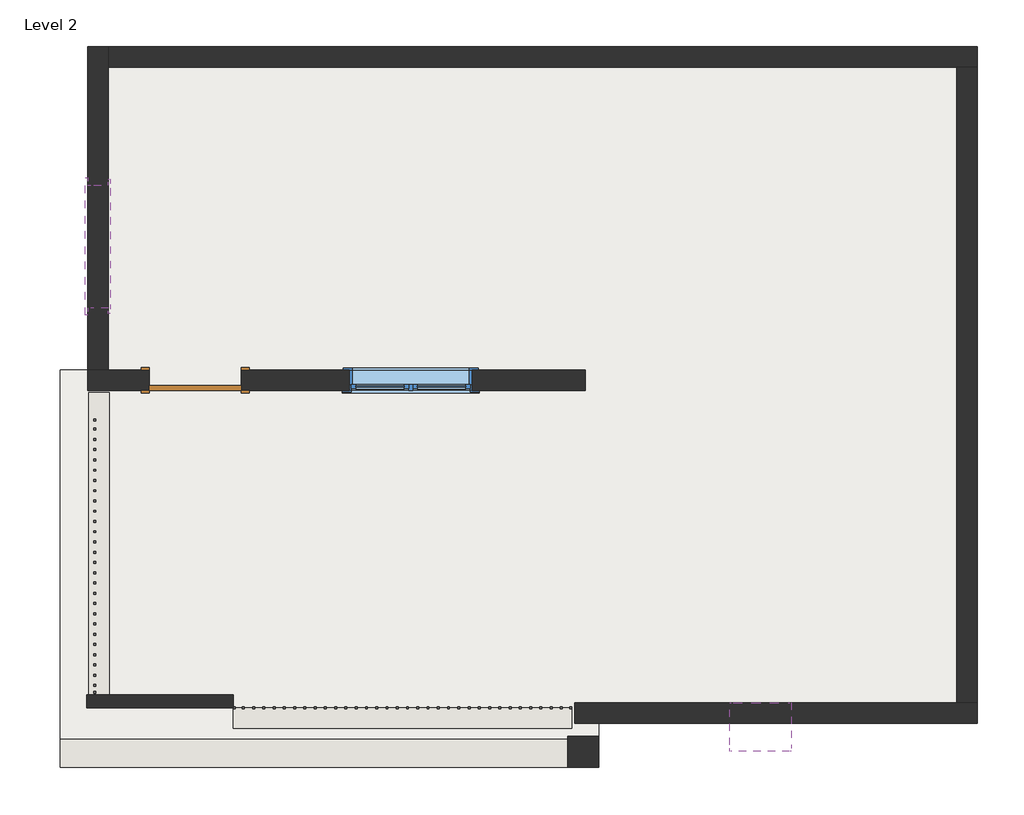
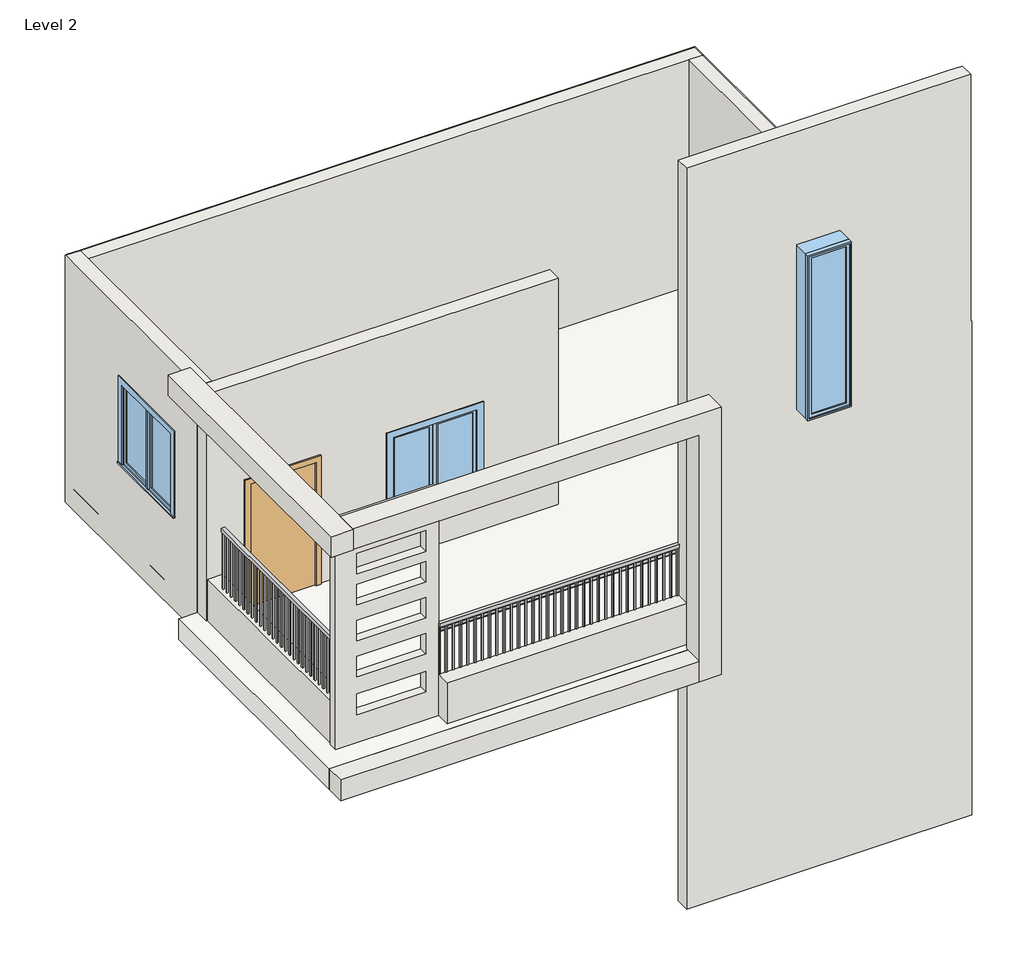
# One storey: 10 walls, 3 windows, 2 railings, 1 door, 1 roof.
"""IFC4 building model written with IfcOpenShell, lengths in millimetres."""

from ifc_helpers import new_model, si_unit, point, frame, frame_2d, origin, place, context, project, spatial, polyline, circle_curve, trimmed, segment, composite_curve, outline, extrude, faceted_brep, transform, mapped, element, save
from components import door_54dd4da4, walls_3_walls_3_b11343c7, walls_4_walls_4_2164e9f1, window_0862ab64, window_a3455bd6

model = new_model("IFC4")

# Units and contexts
model_context = context("Model", 3, world=origin())
ifc_project = project(units=[si_unit("LENGTHUNIT", "METRE", prefix="MILLI")], contexts=[model_context])

# Site, building, storey
site = spatial("IfcSite", under=ifc_project)
building = spatial("IfcBuilding", under=site)
storey = spatial("IfcBuildingStorey", under=building, Name="Level 2", Elevation=3657.6)

# Door
placement = place(None, origin())
door_shape = door_54dd4da4(model_context)
element("IfcDoor", 1, ObjectType="Single-Flush : 36\" x 84\"", at=placement, inside=storey, context=model_context, shape_type="MappedRepresentation", body=[
    mapped(door_shape, transform((-10526.949546, 9086.334124, 3657.6), x_axis=(-1.0, 0.0, 0.0), y_axis=(0.0, -1.0, 0.0), z_axis=(0.0, 0.0, 1.0))),
])

# Railings
element("IfcRailing", 2, ObjectType="Guardrail - Rectangular", at=placement, inside=storey, context=model_context, shape_type="SweptSolid", body=[
    extrude(outline(composite_curve([segment(trimmed(circle_curve(frame_2d((5918.6170892, 5162.55)), 19.05), [point((5899.5670892, 5162.55))], [point((5937.6670892, 5162.55))], False, "CARTESIAN"), True, "CONTINUOUS"), segment(trimmed(circle_curve(frame_2d((5918.6170892, 5162.55)), 19.05), [point((5937.6670892, 5162.55))], [point((5899.5670892, 5162.55))], False, "CARTESIAN"), True, "CONTINUOUS")], self_intersect=False)), frame((-10152.299546, 0.0, 0.0), z_axis=(1.0, 0.0, 0.0), x_axis=(0.0, 1.0, 0.0)), (0.0, 0.0, 1.0), 3352.8),
    extrude(outline(polyline([(-10152.299546, 5817.0170892), (-10152.299546, 5867.8170892), (-6799.499546, 5867.8170892), (-6799.499546, 5817.0170892), (-10152.299546, 5817.0170892)])), frame((0.0, 0.0, 5283.2), z_axis=(0.0, 0.0, 1.0), x_axis=(1.0, 0.0, 0.0)), (0.0, 0.0, 1.0), 50.8),
    extrude(outline(polyline([(-6910.624546, 5832.8920892), (-6910.624546, 5851.9420892), (-6891.574546, 5851.9420892), (-6891.574546, 5832.8920892), (-6910.624546, 5832.8920892)])), frame((0.0, 0.0, 4267.2), z_axis=(0.0, 0.0, 1.0), x_axis=(1.0, 0.0, 0.0)), (0.0, 0.0, 1.0), 1016.0),
    extrude(outline(polyline([(-7012.224546, 5832.8920892), (-7012.224546, 5851.9420892), (-6993.174546, 5851.9420892), (-6993.174546, 5832.8920892), (-7012.224546, 5832.8920892)])), frame((0.0, 0.0, 4267.2), z_axis=(0.0, 0.0, 1.0), x_axis=(1.0, 0.0, 0.0)), (0.0, 0.0, 1.0), 1016.0),
    extrude(outline(polyline([(-7113.824546, 5832.8920892), (-7113.824546, 5851.9420892), (-7094.774546, 5851.9420892), (-7094.774546, 5832.8920892), (-7113.824546, 5832.8920892)])), frame((0.0, 0.0, 4267.2), z_axis=(0.0, 0.0, 1.0), x_axis=(1.0, 0.0, 0.0)), (0.0, 0.0, 1.0), 1016.0),
    extrude(outline(polyline([(-7215.424546, 5832.8920892), (-7215.424546, 5851.9420892), (-7196.374546, 5851.9420892), (-7196.374546, 5832.8920892), (-7215.424546, 5832.8920892)])), frame((0.0, 0.0, 4267.2), z_axis=(0.0, 0.0, 1.0), x_axis=(1.0, 0.0, 0.0)), (0.0, 0.0, 1.0), 1016.0),
    extrude(outline(polyline([(-7317.024546, 5832.8920892), (-7317.024546, 5851.9420892), (-7297.974546, 5851.9420892), (-7297.974546, 5832.8920892), (-7317.024546, 5832.8920892)])), frame((0.0, 0.0, 4267.2), z_axis=(0.0, 0.0, 1.0), x_axis=(1.0, 0.0, 0.0)), (0.0, 0.0, 1.0), 1016.0),
    extrude(outline(polyline([(-7418.624546, 5832.8920892), (-7418.624546, 5851.9420892), (-7399.574546, 5851.9420892), (-7399.574546, 5832.8920892), (-7418.624546, 5832.8920892)])), frame((0.0, 0.0, 4267.2), z_axis=(0.0, 0.0, 1.0), x_axis=(1.0, 0.0, 0.0)), (0.0, 0.0, 1.0), 1016.0),
    extrude(outline(polyline([(-7520.224546, 5832.8920892), (-7520.224546, 5851.9420892), (-7501.174546, 5851.9420892), (-7501.174546, 5832.8920892), (-7520.224546, 5832.8920892)])), frame((0.0, 0.0, 4267.2), z_axis=(0.0, 0.0, 1.0), x_axis=(1.0, 0.0, 0.0)), (0.0, 0.0, 1.0), 1016.0),
    extrude(outline(polyline([(-7621.824546, 5832.8920892), (-7621.824546, 5851.9420892), (-7602.774546, 5851.9420892), (-7602.774546, 5832.8920892), (-7621.824546, 5832.8920892)])), frame((0.0, 0.0, 4267.2), z_axis=(0.0, 0.0, 1.0), x_axis=(1.0, 0.0, 0.0)), (0.0, 0.0, 1.0), 1016.0),
    extrude(outline(polyline([(-7723.424546, 5832.8920892), (-7723.424546, 5851.9420892), (-7704.374546, 5851.9420892), (-7704.374546, 5832.8920892), (-7723.424546, 5832.8920892)])), frame((0.0, 0.0, 4267.2), z_axis=(0.0, 0.0, 1.0), x_axis=(1.0, 0.0, 0.0)), (0.0, 0.0, 1.0), 1016.0),
    extrude(outline(polyline([(-7825.024546, 5832.8920892), (-7825.024546, 5851.9420892), (-7805.974546, 5851.9420892), (-7805.974546, 5832.8920892), (-7825.024546, 5832.8920892)])), frame((0.0, 0.0, 4267.2), z_axis=(0.0, 0.0, 1.0), x_axis=(1.0, 0.0, 0.0)), (0.0, 0.0, 1.0), 1016.0),
    extrude(outline(polyline([(-7926.624546, 5832.8920892), (-7926.624546, 5851.9420892), (-7907.574546, 5851.9420892), (-7907.574546, 5832.8920892), (-7926.624546, 5832.8920892)])), frame((0.0, 0.0, 4267.2), z_axis=(0.0, 0.0, 1.0), x_axis=(1.0, 0.0, 0.0)), (0.0, 0.0, 1.0), 1016.0),
    extrude(outline(polyline([(-8028.224546, 5832.8920892), (-8028.224546, 5851.9420892), (-8009.174546, 5851.9420892), (-8009.174546, 5832.8920892), (-8028.224546, 5832.8920892)])), frame((0.0, 0.0, 4267.2), z_axis=(0.0, 0.0, 1.0), x_axis=(1.0, 0.0, 0.0)), (0.0, 0.0, 1.0), 1016.0),
    extrude(outline(polyline([(-8129.824546, 5832.8920892), (-8129.824546, 5851.9420892), (-8110.774546, 5851.9420892), (-8110.774546, 5832.8920892), (-8129.824546, 5832.8920892)])), frame((0.0, 0.0, 4267.2), z_axis=(0.0, 0.0, 1.0), x_axis=(1.0, 0.0, 0.0)), (0.0, 0.0, 1.0), 1016.0),
    extrude(outline(polyline([(-8231.424546, 5832.8920892), (-8231.424546, 5851.9420892), (-8212.374546, 5851.9420892), (-8212.374546, 5832.8920892), (-8231.424546, 5832.8920892)])), frame((0.0, 0.0, 4267.2), z_axis=(0.0, 0.0, 1.0), x_axis=(1.0, 0.0, 0.0)), (0.0, 0.0, 1.0), 1016.0),
    extrude(outline(polyline([(-8333.024546, 5832.8920892), (-8333.024546, 5851.9420892), (-8313.974546, 5851.9420892), (-8313.974546, 5832.8920892), (-8333.024546, 5832.8920892)])), frame((0.0, 0.0, 4267.2), z_axis=(0.0, 0.0, 1.0), x_axis=(1.0, 0.0, 0.0)), (0.0, 0.0, 1.0), 1016.0),
    extrude(outline(polyline([(-8434.624546, 5832.8920892), (-8434.624546, 5851.9420892), (-8415.574546, 5851.9420892), (-8415.574546, 5832.8920892), (-8434.624546, 5832.8920892)])), frame((0.0, 0.0, 4267.2), z_axis=(0.0, 0.0, 1.0), x_axis=(1.0, 0.0, 0.0)), (0.0, 0.0, 1.0), 1016.0),
    extrude(outline(polyline([(-8536.224546, 5832.8920892), (-8536.224546, 5851.9420892), (-8517.174546, 5851.9420892), (-8517.174546, 5832.8920892), (-8536.224546, 5832.8920892)])), frame((0.0, 0.0, 4267.2), z_axis=(0.0, 0.0, 1.0), x_axis=(1.0, 0.0, 0.0)), (0.0, 0.0, 1.0), 1016.0),
    extrude(outline(polyline([(-8637.824546, 5832.8920892), (-8637.824546, 5851.9420892), (-8618.774546, 5851.9420892), (-8618.774546, 5832.8920892), (-8637.824546, 5832.8920892)])), frame((0.0, 0.0, 4267.2), z_axis=(0.0, 0.0, 1.0), x_axis=(1.0, 0.0, 0.0)), (0.0, 0.0, 1.0), 1016.0),
    extrude(outline(polyline([(-8739.424546, 5832.8920892), (-8739.424546, 5851.9420892), (-8720.374546, 5851.9420892), (-8720.374546, 5832.8920892), (-8739.424546, 5832.8920892)])), frame((0.0, 0.0, 4267.2), z_axis=(0.0, 0.0, 1.0), x_axis=(1.0, 0.0, 0.0)), (0.0, 0.0, 1.0), 1016.0),
    extrude(outline(polyline([(-8841.024546, 5832.8920892), (-8841.024546, 5851.9420892), (-8821.974546, 5851.9420892), (-8821.974546, 5832.8920892), (-8841.024546, 5832.8920892)])), frame((0.0, 0.0, 4267.2), z_axis=(0.0, 0.0, 1.0), x_axis=(1.0, 0.0, 0.0)), (0.0, 0.0, 1.0), 1016.0),
    extrude(outline(polyline([(-8942.624546, 5832.8920892), (-8942.624546, 5851.9420892), (-8923.574546, 5851.9420892), (-8923.574546, 5832.8920892), (-8942.624546, 5832.8920892)])), frame((0.0, 0.0, 4267.2), z_axis=(0.0, 0.0, 1.0), x_axis=(1.0, 0.0, 0.0)), (0.0, 0.0, 1.0), 1016.0),
    extrude(outline(polyline([(-9044.224546, 5832.8920892), (-9044.224546, 5851.9420892), (-9025.174546, 5851.9420892), (-9025.174546, 5832.8920892), (-9044.224546, 5832.8920892)])), frame((0.0, 0.0, 4267.2), z_axis=(0.0, 0.0, 1.0), x_axis=(1.0, 0.0, 0.0)), (0.0, 0.0, 1.0), 1016.0),
    extrude(outline(polyline([(-9145.824546, 5832.8920892), (-9145.824546, 5851.9420892), (-9126.774546, 5851.9420892), (-9126.774546, 5832.8920892), (-9145.824546, 5832.8920892)])), frame((0.0, 0.0, 4267.2), z_axis=(0.0, 0.0, 1.0), x_axis=(1.0, 0.0, 0.0)), (0.0, 0.0, 1.0), 1016.0),
    extrude(outline(polyline([(-9247.424546, 5832.8920892), (-9247.424546, 5851.9420892), (-9228.374546, 5851.9420892), (-9228.374546, 5832.8920892), (-9247.424546, 5832.8920892)])), frame((0.0, 0.0, 4267.2), z_axis=(0.0, 0.0, 1.0), x_axis=(1.0, 0.0, 0.0)), (0.0, 0.0, 1.0), 1016.0),
    extrude(outline(polyline([(-9349.024546, 5832.8920892), (-9349.024546, 5851.9420892), (-9329.974546, 5851.9420892), (-9329.974546, 5832.8920892), (-9349.024546, 5832.8920892)])), frame((0.0, 0.0, 4267.2), z_axis=(0.0, 0.0, 1.0), x_axis=(1.0, 0.0, 0.0)), (0.0, 0.0, 1.0), 1016.0),
    extrude(outline(polyline([(-9450.624546, 5832.8920892), (-9450.624546, 5851.9420892), (-9431.574546, 5851.9420892), (-9431.574546, 5832.8920892), (-9450.624546, 5832.8920892)])), frame((0.0, 0.0, 4267.2), z_axis=(0.0, 0.0, 1.0), x_axis=(1.0, 0.0, 0.0)), (0.0, 0.0, 1.0), 1016.0),
    extrude(outline(polyline([(-9552.224546, 5832.8920892), (-9552.224546, 5851.9420892), (-9533.174546, 5851.9420892), (-9533.174546, 5832.8920892), (-9552.224546, 5832.8920892)])), frame((0.0, 0.0, 4267.2), z_axis=(0.0, 0.0, 1.0), x_axis=(1.0, 0.0, 0.0)), (0.0, 0.0, 1.0), 1016.0),
    extrude(outline(polyline([(-9653.824546, 5832.8920892), (-9653.824546, 5851.9420892), (-9634.774546, 5851.9420892), (-9634.774546, 5832.8920892), (-9653.824546, 5832.8920892)])), frame((0.0, 0.0, 4267.2), z_axis=(0.0, 0.0, 1.0), x_axis=(1.0, 0.0, 0.0)), (0.0, 0.0, 1.0), 1016.0),
    extrude(outline(polyline([(-9755.424546, 5832.8920892), (-9755.424546, 5851.9420892), (-9736.374546, 5851.9420892), (-9736.374546, 5832.8920892), (-9755.424546, 5832.8920892)])), frame((0.0, 0.0, 4267.2), z_axis=(0.0, 0.0, 1.0), x_axis=(1.0, 0.0, 0.0)), (0.0, 0.0, 1.0), 1016.0),
    extrude(outline(polyline([(-9857.024546, 5832.8920892), (-9857.024546, 5851.9420892), (-9837.974546, 5851.9420892), (-9837.974546, 5832.8920892), (-9857.024546, 5832.8920892)])), frame((0.0, 0.0, 4267.2), z_axis=(0.0, 0.0, 1.0), x_axis=(1.0, 0.0, 0.0)), (0.0, 0.0, 1.0), 1016.0),
    extrude(outline(polyline([(-9958.624546, 5832.8920892), (-9958.624546, 5851.9420892), (-9939.574546, 5851.9420892), (-9939.574546, 5832.8920892), (-9958.624546, 5832.8920892)])), frame((0.0, 0.0, 4267.2), z_axis=(0.0, 0.0, 1.0), x_axis=(1.0, 0.0, 0.0)), (0.0, 0.0, 1.0), 1016.0),
    extrude(outline(polyline([(-10060.224546, 5832.8920892), (-10060.224546, 5851.9420892), (-10041.174546, 5851.9420892), (-10041.174546, 5832.8920892), (-10060.224546, 5832.8920892)])), frame((0.0, 0.0, 4267.2), z_axis=(0.0, 0.0, 1.0), x_axis=(1.0, 0.0, 0.0)), (0.0, 0.0, 1.0), 1016.0),
    extrude(outline(polyline([(-6818.549546, 5832.8920892), (-6818.549546, 5851.9420892), (-6799.499546, 5851.9420892), (-6799.499546, 5832.8920892), (-6818.549546, 5832.8920892)])), frame((0.0, 0.0, 4267.2), z_axis=(0.0, 0.0, 1.0), x_axis=(1.0, 0.0, 0.0)), (0.0, 0.0, 1.0), 1016.0),
    extrude(outline(polyline([(-10152.299546, 5832.8920892), (-10152.299546, 5851.9420892), (-10133.249546, 5851.9420892), (-10133.249546, 5832.8920892), (-10152.299546, 5832.8920892)])), frame((0.0, 0.0, 4267.2), z_axis=(0.0, 0.0, 1.0), x_axis=(1.0, 0.0, 0.0)), (0.0, 0.0, 1.0), 1016.0),
])
element("IfcRailing", 3, ObjectType="Handrail - Rectangular", at=placement, inside=storey, context=model_context, shape_type="SweptSolid", body=[
    extrude(outline(polyline([(-11546.3389289, 8704.7828881), (-11495.5389289, 8704.7828881), (-11495.5389289, 5986.9828881), (-11546.3389289, 5986.9828881), (-11546.3389289, 8704.7828881)])), frame((0.0, 0.0, 5435.6), z_axis=(0.0, 0.0, 1.0), x_axis=(1.0, 0.0, 0.0)), (0.0, 0.0, 1.0), 50.8),
    extrude(outline(polyline([(-11530.4639289, 6072.7078881), (-11511.4139289, 6072.7078881), (-11511.4139289, 6053.6578881), (-11530.4639289, 6053.6578881), (-11530.4639289, 6072.7078881)])), frame((0.0, 0.0, 4572.0), z_axis=(0.0, 0.0, 1.0), x_axis=(1.0, 0.0, 0.0)), (0.0, 0.0, 1.0), 863.6),
    extrude(outline(polyline([(-11530.4639289, 6174.3078881), (-11511.4139289, 6174.3078881), (-11511.4139289, 6155.2578881), (-11530.4639289, 6155.2578881), (-11530.4639289, 6174.3078881)])), frame((0.0, 0.0, 4572.0), z_axis=(0.0, 0.0, 1.0), x_axis=(1.0, 0.0, 0.0)), (0.0, 0.0, 1.0), 863.6),
    extrude(outline(polyline([(-11530.4639289, 6275.9078881), (-11511.4139289, 6275.9078881), (-11511.4139289, 6256.8578881), (-11530.4639289, 6256.8578881), (-11530.4639289, 6275.9078881)])), frame((0.0, 0.0, 4572.0), z_axis=(0.0, 0.0, 1.0), x_axis=(1.0, 0.0, 0.0)), (0.0, 0.0, 1.0), 863.6),
    extrude(outline(polyline([(-11530.4639289, 6479.1078881), (-11511.4139289, 6479.1078881), (-11511.4139289, 6460.0578881), (-11530.4639289, 6460.0578881), (-11530.4639289, 6479.1078881)])), frame((0.0, 0.0, 4572.0), z_axis=(0.0, 0.0, 1.0), x_axis=(1.0, 0.0, 0.0)), (0.0, 0.0, 1.0), 863.6),
    extrude(outline(polyline([(-11530.4639289, 6580.7078881), (-11511.4139289, 6580.7078881), (-11511.4139289, 6561.6578881), (-11530.4639289, 6561.6578881), (-11530.4639289, 6580.7078881)])), frame((0.0, 0.0, 4572.0), z_axis=(0.0, 0.0, 1.0), x_axis=(1.0, 0.0, 0.0)), (0.0, 0.0, 1.0), 863.6),
    extrude(outline(polyline([(-11530.4639289, 6682.3078881), (-11511.4139289, 6682.3078881), (-11511.4139289, 6663.2578881), (-11530.4639289, 6663.2578881), (-11530.4639289, 6682.3078881)])), frame((0.0, 0.0, 4572.0), z_axis=(0.0, 0.0, 1.0), x_axis=(1.0, 0.0, 0.0)), (0.0, 0.0, 1.0), 863.6),
    extrude(outline(polyline([(-11530.4639289, 6783.9078881), (-11511.4139289, 6783.9078881), (-11511.4139289, 6764.8578881), (-11530.4639289, 6764.8578881), (-11530.4639289, 6783.9078881)])), frame((0.0, 0.0, 4572.0), z_axis=(0.0, 0.0, 1.0), x_axis=(1.0, 0.0, 0.0)), (0.0, 0.0, 1.0), 863.6),
    extrude(outline(polyline([(-11530.4639289, 6885.5078881), (-11511.4139289, 6885.5078881), (-11511.4139289, 6866.4578881), (-11530.4639289, 6866.4578881), (-11530.4639289, 6885.5078881)])), frame((0.0, 0.0, 4572.0), z_axis=(0.0, 0.0, 1.0), x_axis=(1.0, 0.0, 0.0)), (0.0, 0.0, 1.0), 863.6),
    extrude(outline(polyline([(-11530.4639289, 6987.1078881), (-11511.4139289, 6987.1078881), (-11511.4139289, 6968.0578881), (-11530.4639289, 6968.0578881), (-11530.4639289, 6987.1078881)])), frame((0.0, 0.0, 4572.0), z_axis=(0.0, 0.0, 1.0), x_axis=(1.0, 0.0, 0.0)), (0.0, 0.0, 1.0), 863.6),
    extrude(outline(polyline([(-11530.4639289, 7088.7078881), (-11511.4139289, 7088.7078881), (-11511.4139289, 7069.6578881), (-11530.4639289, 7069.6578881), (-11530.4639289, 7088.7078881)])), frame((0.0, 0.0, 4572.0), z_axis=(0.0, 0.0, 1.0), x_axis=(1.0, 0.0, 0.0)), (0.0, 0.0, 1.0), 863.6),
    extrude(outline(polyline([(-11530.4639289, 7190.3078881), (-11511.4139289, 7190.3078881), (-11511.4139289, 7171.2578881), (-11530.4639289, 7171.2578881), (-11530.4639289, 7190.3078881)])), frame((0.0, 0.0, 4572.0), z_axis=(0.0, 0.0, 1.0), x_axis=(1.0, 0.0, 0.0)), (0.0, 0.0, 1.0), 863.6),
    extrude(outline(polyline([(-11530.4639289, 7291.9078881), (-11511.4139289, 7291.9078881), (-11511.4139289, 7272.8578881), (-11530.4639289, 7272.8578881), (-11530.4639289, 7291.9078881)])), frame((0.0, 0.0, 4572.0), z_axis=(0.0, 0.0, 1.0), x_axis=(1.0, 0.0, 0.0)), (0.0, 0.0, 1.0), 863.6),
    extrude(outline(polyline([(-11530.4639289, 7393.5078881), (-11511.4139289, 7393.5078881), (-11511.4139289, 7374.4578881), (-11530.4639289, 7374.4578881), (-11530.4639289, 7393.5078881)])), frame((0.0, 0.0, 4572.0), z_axis=(0.0, 0.0, 1.0), x_axis=(1.0, 0.0, 0.0)), (0.0, 0.0, 1.0), 863.6),
    extrude(outline(polyline([(-11530.4639289, 7495.1078881), (-11511.4139289, 7495.1078881), (-11511.4139289, 7476.0578881), (-11530.4639289, 7476.0578881), (-11530.4639289, 7495.1078881)])), frame((0.0, 0.0, 4572.0), z_axis=(0.0, 0.0, 1.0), x_axis=(1.0, 0.0, 0.0)), (0.0, 0.0, 1.0), 863.6),
    extrude(outline(polyline([(-11530.4639289, 7596.7078881), (-11511.4139289, 7596.7078881), (-11511.4139289, 7577.6578881), (-11530.4639289, 7577.6578881), (-11530.4639289, 7596.7078881)])), frame((0.0, 0.0, 4572.0), z_axis=(0.0, 0.0, 1.0), x_axis=(1.0, 0.0, 0.0)), (0.0, 0.0, 1.0), 863.6),
    extrude(outline(polyline([(-11530.4639289, 7698.3078881), (-11511.4139289, 7698.3078881), (-11511.4139289, 7679.2578881), (-11530.4639289, 7679.2578881), (-11530.4639289, 7698.3078881)])), frame((0.0, 0.0, 4572.0), z_axis=(0.0, 0.0, 1.0), x_axis=(1.0, 0.0, 0.0)), (0.0, 0.0, 1.0), 863.6),
    extrude(outline(polyline([(-11530.4639289, 7799.9078881), (-11511.4139289, 7799.9078881), (-11511.4139289, 7780.8578881), (-11530.4639289, 7780.8578881), (-11530.4639289, 7799.9078881)])), frame((0.0, 0.0, 4572.0), z_axis=(0.0, 0.0, 1.0), x_axis=(1.0, 0.0, 0.0)), (0.0, 0.0, 1.0), 863.6),
    extrude(outline(polyline([(-11530.4639289, 7901.5078881), (-11511.4139289, 7901.5078881), (-11511.4139289, 7882.4578881), (-11530.4639289, 7882.4578881), (-11530.4639289, 7901.5078881)])), frame((0.0, 0.0, 4572.0), z_axis=(0.0, 0.0, 1.0), x_axis=(1.0, 0.0, 0.0)), (0.0, 0.0, 1.0), 863.6),
    extrude(outline(polyline([(-11530.4639289, 8003.1078881), (-11511.4139289, 8003.1078881), (-11511.4139289, 7984.0578881), (-11530.4639289, 7984.0578881), (-11530.4639289, 8003.1078881)])), frame((0.0, 0.0, 4572.0), z_axis=(0.0, 0.0, 1.0), x_axis=(1.0, 0.0, 0.0)), (0.0, 0.0, 1.0), 863.6),
    extrude(outline(polyline([(-11530.4639289, 8104.7078881), (-11511.4139289, 8104.7078881), (-11511.4139289, 8085.6578881), (-11530.4639289, 8085.6578881), (-11530.4639289, 8104.7078881)])), frame((0.0, 0.0, 4572.0), z_axis=(0.0, 0.0, 1.0), x_axis=(1.0, 0.0, 0.0)), (0.0, 0.0, 1.0), 863.6),
    extrude(outline(polyline([(-11530.4639289, 8206.3078881), (-11511.4139289, 8206.3078881), (-11511.4139289, 8187.2578881), (-11530.4639289, 8187.2578881), (-11530.4639289, 8206.3078881)])), frame((0.0, 0.0, 4572.0), z_axis=(0.0, 0.0, 1.0), x_axis=(1.0, 0.0, 0.0)), (0.0, 0.0, 1.0), 863.6),
    extrude(outline(polyline([(-11530.4639289, 8307.9078881), (-11511.4139289, 8307.9078881), (-11511.4139289, 8288.8578881), (-11530.4639289, 8288.8578881), (-11530.4639289, 8307.9078881)])), frame((0.0, 0.0, 4572.0), z_axis=(0.0, 0.0, 1.0), x_axis=(1.0, 0.0, 0.0)), (0.0, 0.0, 1.0), 863.6),
    extrude(outline(polyline([(-11530.4639289, 8409.5078881), (-11511.4139289, 8409.5078881), (-11511.4139289, 8390.4578881), (-11530.4639289, 8390.4578881), (-11530.4639289, 8409.5078881)])), frame((0.0, 0.0, 4572.0), z_axis=(0.0, 0.0, 1.0), x_axis=(1.0, 0.0, 0.0)), (0.0, 0.0, 1.0), 863.6),
    extrude(outline(polyline([(-11530.4639289, 8511.1078881), (-11511.4139289, 8511.1078881), (-11511.4139289, 8492.0578881), (-11530.4639289, 8492.0578881), (-11530.4639289, 8511.1078881)])), frame((0.0, 0.0, 4572.0), z_axis=(0.0, 0.0, 1.0), x_axis=(1.0, 0.0, 0.0)), (0.0, 0.0, 1.0), 863.6),
    extrude(outline(polyline([(-11530.4639289, 8612.7078881), (-11511.4139289, 8612.7078881), (-11511.4139289, 8593.6578881), (-11530.4639289, 8593.6578881), (-11530.4639289, 8612.7078881)])), frame((0.0, 0.0, 4572.0), z_axis=(0.0, 0.0, 1.0), x_axis=(1.0, 0.0, 0.0)), (0.0, 0.0, 1.0), 863.6),
    extrude(outline(polyline([(-11530.4639289, 6377.5078881), (-11511.4139289, 6377.5078881), (-11511.4139289, 6358.4578881), (-11530.4639289, 6358.4578881), (-11530.4639289, 6377.5078881)])), frame((0.0, 0.0, 4572.0), z_axis=(0.0, 0.0, 1.0), x_axis=(1.0, 0.0, 0.0)), (0.0, 0.0, 1.0), 863.6),
    extrude(outline(polyline([(-11530.4639289, 6006.0328881), (-11511.4139289, 6006.0328881), (-11511.4139289, 5986.9828881), (-11530.4639289, 5986.9828881), (-11530.4639289, 6006.0328881)])), frame((0.0, 0.0, 4572.0), z_axis=(0.0, 0.0, 1.0), x_axis=(1.0, 0.0, 0.0)), (0.0, 0.0, 1.0), 863.6),
    extrude(outline(polyline([(-11530.4639289, 8704.7828881), (-11511.4139289, 8704.7828881), (-11511.4139289, 8685.7328881), (-11530.4639289, 8685.7328881), (-11530.4639289, 8704.7828881)])), frame((0.0, 0.0, 4572.0), z_axis=(0.0, 0.0, 1.0), x_axis=(1.0, 0.0, 0.0)), (0.0, 0.0, 1.0), 863.6),
])

# Roof
element("IfcRoof", 4, ObjectType="Generic - 12\"", at=placement, inside=storey, context=model_context, shape_type="SweptSolid", body=[
    extrude(outline(polyline([(-11593.749546, 12388.334124), (-2789.0236868, 12388.334124), (-2789.0236868, 5893.2170892), (-6529.1736868, 5893.2170892), (-6529.1736868, 5530.334124), (-11863.1736868, 5530.334124), (-11863.1736868, 9187.934124), (-11593.749546, 9187.934124), (-11593.749546, 12388.334124)])), frame((0.0, 0.0, 3657.6), z_axis=(0.0, 0.0, 1.0), x_axis=(1.0, 0.0, 0.0)), (0.0, 0.0, 1.0), 304.8),
])

# Walls
element("IfcWall", 5, ObjectType="Generic - 5\"", at=placement, inside=storey, context=model_context, shape_type="Brep", body=[
    faceted_brep([(-11600.099546, 5842.4170892, 3657.6), (-10152.299546, 5842.4170892, 3657.6), (-10152.299546, 5842.4170892, 7315.2), (-11600.099546, 5842.4170892, 7315.2), (-10331.7856202, 5842.4170892, 6762.7736513), (-10331.7856202, 5842.4170892, 6457.9736513), (-11296.9856202, 5842.4170892, 6457.9736513), (-11296.9856202, 5842.4170892, 6762.7736513), (-10331.7856202, 5842.4170892, 6305.5736513), (-10331.7856202, 5842.4170892, 6000.7736513), (-11296.9856202, 5842.4170892, 6000.7736513), (-11296.9856202, 5842.4170892, 6305.5736513), (-10331.7856202, 5842.4170892, 5772.1736513), (-10331.7856202, 5842.4170892, 5467.3736513), (-11296.9856202, 5842.4170892, 5467.3736513), (-11296.9856202, 5842.4170892, 5772.1736513), (-10331.7856202, 5842.4170892, 5238.7736513), (-10331.7856202, 5842.4170892, 4933.9736513), (-11296.9856202, 5842.4170892, 4933.9736513), (-11296.9856202, 5842.4170892, 5238.7736513), (-10331.7856202, 5842.4170892, 4679.9736513), (-10331.7856202, 5842.4170892, 4375.1736513), (-11296.9856202, 5842.4170892, 4375.1736513), (-11296.9856202, 5842.4170892, 4679.9736513), (-11600.099546, 5969.4170892, 3657.6), (-11600.099546, 5969.4170892, 7315.2), (-10152.299546, 5969.4170892, 7315.2), (-10152.299546, 5969.4170892, 3657.6), (-11377.849546, 5969.4170892, 3657.6), (-11581.049546, 5969.4170892, 3657.6), (-10331.7856202, 5969.4170892, 6762.7736513), (-11296.9856202, 5969.4170892, 6762.7736513), (-11296.9856202, 5969.4170892, 6457.9736513), (-10331.7856202, 5969.4170892, 6457.9736513), (-10331.7856202, 5969.4170892, 6305.5736513), (-11296.9856202, 5969.4170892, 6305.5736513), (-11296.9856202, 5969.4170892, 6000.7736513), (-10331.7856202, 5969.4170892, 6000.7736513), (-10331.7856202, 5969.4170892, 5772.1736513), (-11296.9856202, 5969.4170892, 5772.1736513), (-11296.9856202, 5969.4170892, 5467.3736513), (-10331.7856202, 5969.4170892, 5467.3736513), (-10331.7856202, 5969.4170892, 5238.7736513), (-11296.9856202, 5969.4170892, 5238.7736513), (-11296.9856202, 5969.4170892, 4933.9736513), (-10331.7856202, 5969.4170892, 4933.9736513), (-10331.7856202, 5969.4170892, 4679.9736513), (-11296.9856202, 5969.4170892, 4679.9736513), (-11296.9856202, 5969.4170892, 4375.1736513), (-10331.7856202, 5969.4170892, 4375.1736513)], [[[0, 1, 2, 3], [4, 5, 6, 7], [8, 9, 10, 11], [12, 13, 14, 15], [16, 17, 18, 19], [20, 21, 22, 23]], [[24, 25, 26, 27, 28, 29], [30, 31, 32, 33], [34, 35, 36, 37], [38, 39, 40, 41], [42, 43, 44, 45], [46, 47, 48, 49]], [[1, 0, 24, 29, 28, 27]], [[2, 1, 27, 26]], [[3, 2, 26, 25]], [[0, 3, 25, 24]], [[5, 4, 30, 33]], [[6, 5, 33, 32]], [[7, 6, 32, 31]], [[4, 7, 31, 30]], [[9, 8, 34, 37]], [[10, 9, 37, 36]], [[11, 10, 36, 35]], [[8, 11, 35, 34]], [[13, 12, 38, 41]], [[14, 13, 41, 40]], [[15, 14, 40, 39]], [[12, 15, 39, 38]], [[17, 16, 42, 45]], [[18, 17, 45, 44]], [[19, 18, 44, 43]], [[16, 19, 43, 42]], [[21, 20, 46, 49]], [[22, 21, 49, 48]], [[23, 22, 48, 47]], [[20, 23, 47, 46]]]),
])
element("IfcWall", 6, ObjectType="Generic - 8\"", at=placement, inside=storey, context=model_context, shape_type="Brep", body=[
    faceted_brep([(-11390.549546, 9195.2170892, 3657.6), (-11390.549546, 12192.4170892, 3657.6), (-11390.549546, 12395.6170892, 3657.6), (-11390.549546, 12395.6170892, 7315.2), (-11390.549546, 12388.334124, 7315.2), (-11390.549546, 12192.4170892, 7315.2), (-11390.549546, 9195.2170892, 7315.2), (-11390.549546, 11024.0170892, 6250.2570536), (-11390.549546, 11024.0170892, 5031.0570536), (-11390.549546, 9804.8170892, 5031.0570536), (-11390.549546, 9804.8170892, 6250.2570536), (-11593.749546, 9195.2170892, 3657.6), (-11593.749546, 9195.2170892, 7315.2), (-11593.749546, 12388.334124, 7315.2), (-11593.749546, 12395.6170892, 7315.2), (-11593.749546, 12395.6170892, 3657.6), (-11593.749546, 11024.0170892, 6250.2570536), (-11593.749546, 9804.8170892, 6250.2570536), (-11593.749546, 9804.8170892, 5031.0570536), (-11593.749546, 11024.0170892, 5031.0570536), (-11568.349546, 12395.6170892, 3657.6), (-11568.349546, 12395.6170892, 7315.2)], [[[0, 1, 2, 3, 4, 5, 6], [7, 8, 9, 10]], [[11, 12, 13, 14, 15], [16, 17, 18, 19]], [[2, 1, 0, 11, 15, 20]], [[0, 6, 12, 11]], [[3, 2, 20, 15, 14, 21]], [[4, 3, 21, 14, 13]], [[6, 5, 4, 13, 12]], [[8, 7, 16, 19]], [[9, 8, 19, 18]], [[10, 9, 18, 17]], [[7, 10, 17, 16]]]),
])
element("IfcWall", 7, ObjectType="Generic - 8\"", at=placement, inside=storey, context=model_context, shape_type="Brep", body=[
    faceted_brep([(-11390.549546, 12192.4170892, 3657.6), (-2983.149546, 12192.4170892, 3657.6), (-2779.949546, 12192.4170892, 3657.6), (-2779.949546, 12192.4170892, 7315.2), (-2789.0236868, 12192.4170892, 7315.2), (-2983.149546, 12192.4170892, 7315.2), (-11390.549546, 12192.4170892, 7315.2), (-11390.549546, 12395.6170892, 3657.6), (-11390.549546, 12395.6170892, 7315.2), (-2789.0236868, 12395.6170892, 7315.2), (-2779.949546, 12395.6170892, 7315.2), (-2779.949546, 12395.6170892, 3657.6), (-11390.549546, 12388.334124, 7315.2), (-2779.949546, 12388.334124, 7315.2), (-2789.0236868, 12388.334124, 7315.2)], [[[0, 1, 2, 3, 4, 5, 6]], [[7, 8, 9, 10, 11]], [[2, 1, 0, 7, 11]], [[0, 6, 12, 8, 7]], [[3, 2, 11, 10, 13]], [[4, 3, 13, 14]], [[9, 8, 12, 14]], [[13, 10, 9, 14]], [[6, 5, 4, 14, 12]]]),
])
element("IfcWall", 8, ObjectType="Generic - 8\"", at=placement, inside=storey, context=model_context, shape_type="Brep", body=[
    faceted_brep([(-2983.149546, 12192.4170892, 3657.6), (-2983.149546, 5994.8170892, 3657.6), (-2983.149546, 5893.2170892, 3657.6), (-2983.149546, 5893.2170892, 7315.2), (-2983.149546, 12192.4170892, 7315.2), (-2779.949546, 12192.4170892, 3657.6), (-2779.949546, 12192.4170892, 7315.2), (-2779.949546, 5893.2170892, 7315.2), (-2779.949546, 5893.2170892, 3657.6), (-2779.949546, 5994.8170892, 3657.6), (-2789.0236868, 12192.4170892, 7315.2), (-2789.0236868, 5893.2170892, 7315.2)], [[[0, 1, 2, 3, 4]], [[5, 6, 7, 8, 9]], [[2, 1, 0, 5, 9, 8]], [[0, 4, 10, 6, 5]], [[3, 2, 8, 7, 11]], [[11, 7, 6, 10]], [[4, 3, 11, 10]]]),
])
element("IfcWall", 9, ObjectType="Generic - 8\"", at=placement, inside=storey, context=model_context, shape_type="Brep", body=[
    faceted_brep([(-6767.749546, 5690.0170892, 0.0), (-2779.949546, 5690.0170892, 0.0), (-2779.949546, 5690.0170892, 7315.2), (-2789.0236868, 5690.0170892, 7315.2), (-2789.0236868, 5690.0170892, 10972.8), (-6767.749546, 5690.0170892, 10972.8), (-6767.749546, 5893.2170892, 0.0), (-6767.749546, 5893.2170892, 3657.6), (-6767.749546, 5893.2170892, 10972.8), (-2992.2236868, 5893.2170892, 10972.8), (-2789.0236868, 5893.2170892, 10972.8), (-2789.0236868, 5893.2170892, 7315.2), (-2779.949546, 5893.2170892, 7315.2), (-2779.949546, 5893.2170892, 3657.6), (-2779.949546, 5893.2170892, 0.0), (-6564.549546, 5893.2170892, 0.0)], [[[0, 1, 2, 3, 4, 5]], [[6, 7, 8, 9, 10, 11, 12, 13, 14, 15]], [[1, 0, 6, 15, 14]], [[0, 5, 8, 7, 6]], [[11, 3, 2, 12]], [[2, 1, 14, 13, 12]], [[4, 3, 11, 10]], [[5, 4, 10, 9, 8]]]),
])
element("IfcWall", 10, ObjectType="Generic - 8\"", at=placement, inside=storey, context=model_context, shape_type="SweptSolid", body=[
    extrude(outline(polyline([(3657.6, -11593.749546), (3657.6, -10984.149546), (5791.2, -10984.149546), (5791.2, -10069.749546), (3657.6, -10069.749546), (3657.6, -6666.149546), (7315.2, -6666.149546), (7315.2, -11593.749546), (3657.6, -11593.749546)]), holes=[polyline([(5791.2, -9002.949546), (5791.2, -7783.749546), (4572.0, -7783.749546), (4572.0, -9002.949546), (5791.2, -9002.949546)])]), frame((0.0, 8984.734124, 0.0), z_axis=(0.0, 1.0, 0.0), x_axis=(0.0, 0.0, 1.0)), (0.0, 0.0, 1.0), 203.2),
])
element("IfcWall", 11, ObjectType="Generic - 8\"", at=placement, inside=storey, context=model_context, shape_type="SweptSolid", body=[
    extrude(outline(polyline([(-11581.049546, 5969.4170892), (-11581.049546, 8965.684124), (-11377.849546, 8965.684124), (-11377.849546, 5969.4170892), (-11581.049546, 5969.4170892)])), frame((0.0, 0.0, 3657.6), z_axis=(0.0, 0.0, 1.0), x_axis=(1.0, 0.0, 0.0)), (0.0, 0.0, 1.0), 927.7555883),
])
element("IfcWall", 12, ObjectType="Generic - 8\"", at=placement, inside=storey, context=model_context, shape_type="SweptSolid", body=[
    extrude(outline(polyline([(-6799.499546, 5639.2170892), (-10152.299546, 5639.2170892), (-10152.299546, 5842.4170892), (-6799.499546, 5842.4170892), (-6799.499546, 5639.2170892)])), frame((0.0, 0.0, 3657.6), z_axis=(0.0, 0.0, 1.0), x_axis=(1.0, 0.0, 0.0)), (0.0, 0.0, 1.0), 914.4),
])
walls_3_walls_3_shape = walls_3_walls_3_b11343c7(model_context)
element("IfcWall", 13, ObjectType="Walls 3 : Walls 3", at=placement, inside=storey, context=model_context, shape_type="MappedRepresentation", body=[
    mapped(walls_3_walls_3_shape, transform((0.0, 0.0, 0.0), x_axis=(1.0, 0.0, 0.0), y_axis=(0.0, 1.0, 0.0), z_axis=(0.0, 0.0, 1.0))),
])
walls_4_walls_4_shape = walls_4_walls_4_2164e9f1(model_context)
element("IfcWall", 14, ObjectType="Walls 4 : Walls 4", at=placement, inside=storey, context=model_context, shape_type="MappedRepresentation", body=[
    mapped(walls_4_walls_4_shape, transform((0.0, 0.0, 0.0), x_axis=(1.0, 0.0, 0.0), y_axis=(0.0, 1.0, 0.0), z_axis=(0.0, 0.0, 1.0))),
])

# Windows
window_shape = window_0862ab64(model_context)
element("IfcWindow", 15, ObjectType="Casement Dbl with Trim : 48\" x 48\"", at=placement, inside=storey, context=model_context, shape_type="MappedRepresentation", body=[
    mapped(window_shape, transform((-8393.349546, 9105.384124, 3657.6), x_axis=(-1.0, 0.0, 0.0), y_axis=(0.0, -1.0, 0.0), z_axis=(0.0, 0.0, 1.0))),
])
element("IfcWindow", 16, ObjectType="Casement Dbl with Trim : 48\" x 48\"", at=placement, inside=storey, context=model_context, shape_type="MappedRepresentation", body=[
    mapped(window_shape, transform((-11473.099546, 10414.4170892, 4116.6570536), x_axis=(0.0, 1.0, 0.0), y_axis=(-1.0, 0.0, 0.0), z_axis=(0.0, 0.0, 1.0))),
])
window_2_shape = window_a3455bd6(model_context)
element("IfcWindow", 17, ObjectType="Fixed : 24\" x 96\"", at=placement, inside=storey, context=model_context, shape_type="MappedRepresentation", body=[
    mapped(window_2_shape, transform((-4966.0322745, 5652.0001581, 6561.5811024), x_axis=(-1.0, 0.0, 0.0), y_axis=(0.0, -1.0, 0.0), z_axis=(0.0, 0.0, 1.0))),
])

save(model, "model.ifc")

# Revit data of these elements
# Type "Single-Flush : 36\" x 84\""
#   Type Mark = "1"
#   Construction Type Id = "MDOOR"
#   Assembly Code = "C1020"
#   Analytic Construction = "Metal"
#   Thickness = 0' - 2"
#   Heat Transfer Coefficient (U) = 0.651978 BTU/(h·ft²·°F)
#   Height = 7' - 0"
#   Trim Projection Ext = 0' - 1"
#   Trim Projection Int = 0' - 1"
#   Trim Width = 0' - 3"
#   Width = 3' - 0"
#   Define Thermal Properties by = 1
#   Door Material = Door - Panel
#   Frame Material = Door - Frame
#   Visual Light Transmittance = 0
#   Solar Heat Gain Coefficient = 0
#   Function = (empty or 0)
#   Wall Closure = (empty or 0)
# Type "Guardrail - Rectangular"
#   Assembly Code = "C2010400"
#   built-in parameter 1008612 = 0.0416667 (stored number, unit not read)
#   built-in parameter 1008611 = 0.0416667 (stored number, unit not read)
#   built-in parameter 1008609 = 0.333333 (stored number, unit not read)
#   built-in parameter 1008604 = 0.166667 (stored number, unit not read)
#   built-in parameter 1008603 = 0.166667 (stored number, unit not read)
#   Railing Height = 3' - 6"
#   built-in parameter 1008630 = 2
#   built-in parameter 1008610 = 1
#   built-in parameter 1008618 = Baluster - Square : 3/4"
# Type "Handrail - Rectangular"
#   Assembly Code = "C2010400"
#   built-in parameter 1008612 = 0.0416667 (stored number, unit not read)
#   built-in parameter 1008611 = 0.0416667 (stored number, unit not read)
#   built-in parameter 1008609 = 0.333333 (stored number, unit not read)
#   built-in parameter 1008604 = 0.166667 (stored number, unit not read)
#   built-in parameter 1008603 = 0.166667 (stored number, unit not read)
#   Railing Height = 3' - 0"
#   built-in parameter 1008630 = 2
#   built-in parameter 1008610 = 2
#   built-in parameter 1008618 = Baluster - Square : 3/4"
# Type "Generic - 12\""
#   Assembly Code = "B1020"
#   Layers, outside or top first: 1' - 0" no material (function 1)
# Type "Generic - 5\""
#   Assembly Code = "B2010"
#   Layers, outside or top first: 0' - 5" no material (function 1)
# Type "Generic - 8\""
#   Assembly Code = "B2010"
#   Layers, outside or top first: 0' - 8" no material (function 1)
# Type "Casement Dbl with Trim : 48\" x 48\""
#   Type Mark = "10"
#   Construction Type Id = "GSP4R"
#   Assembly Code = "B2020100"
#   Analytic Construction = "1/8 in Pilkington single glazing"
#   Visual Light Transmittance = 0.9
#   Thermal Resistance (R) = 1.53941 (h·ft²·°F)/BTU
#   Solar Heat Gain Coefficient = 0.78
#   Heat Transfer Coefficient (U) = 0.6496 BTU/(h·ft²·°F)
#   Height = 4' - 0"
#   Default Sill Height = 3' - 0"
#   Trim Projection - Ext. = 0' - 0 1/2"
#   Trim Projection - Int. = 0' - 0 3/4"
#   Trim Width - Exterior = 0' - 3 1/2"
#   Trim Width - Interior = 0' - 3 1/2"
#   Width = 4' - 0"
#   Window Inset = 0' - 0 3/4"
#   Define Thermal Properties by = 1
#   Glass Pane Material = Glass
#   Sash Material = Sash
#   Trim Exterior Material = Trim
#   Trim Interior Material = Trim
#   Wall Closure = (empty or 0)
# Type "Fixed : 24\" x 96\""
#   Type Mark = "6"
#   Construction Type Id = "GSP4R"
#   Assembly Code = "B2020100"
#   Analytic Construction = "1/8 in Pilkington single glazing"
#   Visual Light Transmittance = 0.9
#   Solar Heat Gain Coefficient = 0.78
#   Heat Transfer Coefficient (U) = 0.6496 BTU/(h·ft²·°F)
#   Height = 8' - 0"
#   Default Sill Height = 1' - 0"
#   Width = 2' - 0"
#   Window Inset = 0' - 0 3/4"
#   Define Thermal Properties by = 1
#   Glass Pane Material = Glass
#   Sash Material = Sash
#   Wall Closure = (empty or 0)
# Element 1 (IfcDoor, "Single-Flush : 36\" x 84\"")
#   Phase Created = New Construction
#   Materials on its faces: "Door - Frame", "Door - Panel"
# Element 2 (IfcRailing, "Guardrail - Rectangular")
#   built-in parameter 1008621 = 2 (stored number, unit not read)
#   Phase Created = New Construction
# Element 3 (IfcRailing, "Handrail - Rectangular")
#   built-in parameter 1008621 = 3 (stored number, unit not read)
#   Phase Created = New Construction
# Element 4 (IfcRoof, "Generic - 12\"")
#   built-in parameter 1001705 = 13 (stored number, unit not read)
#   built-in parameter 1001710 = 33615
#   Phase Created = New Construction
#   Materials on its faces: "Default Roof"
# Element 5 (IfcWall, "Generic - 5\"")
#   Top Offset = 0' - 0"
#   Base Offset = 0' - 0"
#   wall height = 12' - 0"
#   Phase Created = New Construction
#   Base Constraint = Level 2
#   Top Constraint = Level 3
#   Materials on its faces: "Default Wall"
# Elements 6, 7, 8, 10 (IfcWall, "Generic - 8\"")
#   Top Offset = 0' - 0"
#   Base Offset = 0' - 0"
#   Unconnected Height = 12' - 0"
#   wall height = 12' - 0"
#   Phase Created = New Construction
#   Base Constraint = Level 2
#   Materials on its faces: "Default Wall"
# Element 9 (IfcWall, "Generic - 8\"")
#   built-in parameter 1001111 = -12' - 0"
#   Top Offset = 0' - 0"
#   Base Offset = -12' - 0"
#   Unconnected Height = 36' - 0"
#   wall height = 36' - 0"
#   Phase Created = New Construction
#   Base Constraint = Level 2
#   Materials on its faces: "Default Wall"
# Element 11 (IfcWall, "Generic - 8\"")
#   Top Offset = 0' - 0"
#   Base Offset = 0' - 0"
#   Unconnected Height = 3' - 0.52581"
#   wall height = 3' - 0.52581"
#   Phase Created = New Construction
#   Base Constraint = Level 2
#   Materials on its faces: "Default Wall"
# Element 12 (IfcWall, "Generic - 8\"")
#   Top Offset = 0' - 0"
#   Base Offset = 0' - 0"
#   Unconnected Height = 3' - 0"
#   wall height = 3' - 0"
#   Phase Created = New Construction
#   Base Constraint = Level 2
#   Materials on its faces: "Default Wall"
# Element 13 (IfcWall, "Walls 3 : Walls 3")
#   Phase Created = New Construction
#   Materials on its faces: "Default Wall"
# Element 14 (IfcWall, "Walls 4 : Walls 4")
#   Phase Created = New Construction
#   Materials on its faces: "Default Wall"
# Element 15 (IfcWindow, "Casement Dbl with Trim : 48\" x 48\"")
#   Mark = "1"
#   Phase Created = New Construction
#   Materials on its faces: "Sash", "Trim", "Glass"
# Element 16 (IfcWindow, "Casement Dbl with Trim : 48\" x 48\"")
#   Mark = "3"
#   Phase Created = New Construction
#   Materials on its faces: "Sash", "Trim", "Glass"
# Element 17 (IfcWindow, "Fixed : 24\" x 96\"")
#   Mark = "5"
#   Phase Created = New Construction
#   Materials on its faces: "Sash", "Glass"
# Materials
#   "Door - Panel": class "Wood", colour RGB 210 159 95, transparency 0
#   "Door - Frame": colour RGB 118 70 51, transparency 0
#   "Glass": class "Glass", colour RGB 0 128 192, transparency 0.75, Description = "Soda Lime Glass", Cost = 0
#   "Sash": class "Wood", colour RGB 224 178 126, transparency 0
#   "Trim": class "Wood", colour RGB 224 178 126, transparency 0
#   "Default Roof": colour RGB 88 101 114, transparency 0
#   "Default Wall": colour RGB 128 128 128, transparency 0
